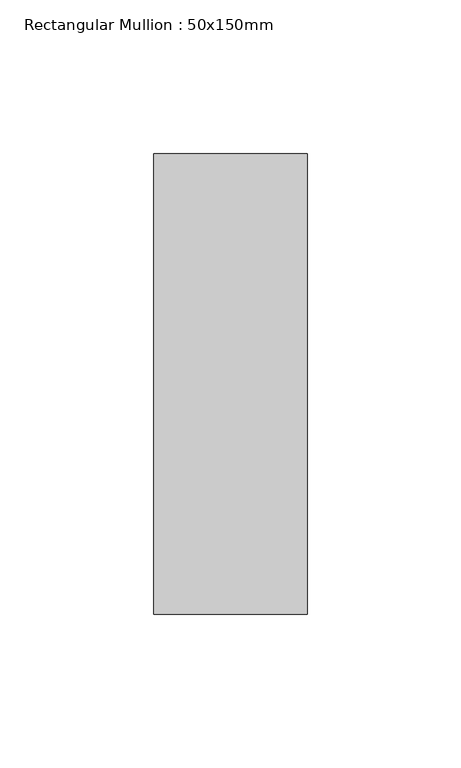
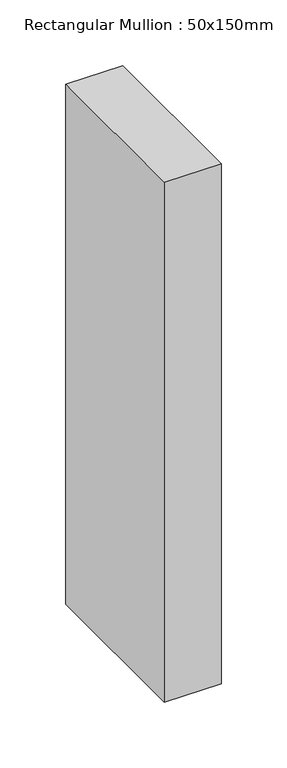
"""IFC4 building model written with IfcOpenShell, lengths in millimetres: member geometry, Rectangular Mullion : 50x150mm."""

from ifc_helpers import new_model, si_unit, frame, origin, place, context, project, spatial, polyline, outline, extrude, source, transform, mapped, element, save


def rectangular_mullion_50x150mm_b9b5507c(model_context):
    return source(origin(), model_context, "Body", "SweptSolid", [
        extrude(outline(polyline([(0.0, 75.0), (0.0, -75.0), (-50.0, -75.0), (-50.0, 75.0), (0.0, 75.0)])), frame((0.0, 0.0, -483.4), z_axis=(0.0, 0.0, 1.0), x_axis=(1.0, 0.0, 0.0)), (0.0, 0.0, 1.0), 483.4),
    ])


if __name__ == "__main__":
    model = new_model("IFC4")
    model_context = context("Model", 3, world=origin())
    ifc_project = project(units=[si_unit("LENGTHUNIT", "METRE", prefix="MILLI")], contexts=[model_context])
    site = spatial("IfcSite", under=ifc_project)
    building = spatial("IfcBuilding", under=site)
    placement = place(None, origin())
    rectangular_mullion_50x150mm_shape = rectangular_mullion_50x150mm_b9b5507c(model_context)
    element("IfcMember", 1, ObjectType="Rectangular Mullion : 50x150mm", at=placement, inside=building, context=model_context, shape_type="MappedRepresentation", body=[
        mapped(rectangular_mullion_50x150mm_shape, transform((0.0, 0.0, 0.0), x_axis=(1.0, 0.0, 0.0), y_axis=(0.0, 1.0, 0.0), z_axis=(0.0, 0.0, 1.0))),
    ])
    save(model, "model.ifc")

# Revit data of these elements
# Type "Rectangular Mullion : 50x150mm"
#   Keynote = "H11"
#   built-in parameter 1007304 = 0.492126 (stored number, unit not read)
#   built-in parameter 1007301 = 0.082021 (stored number, unit not read)
#   built-in parameter 1007300 = 0.082021 (stored number, unit not read)
# Element 1 (IfcMember, "Rectangular Mullion : 50x150mm")
#   Materials on its faces: "Aluminium"
# Materials
#   "Aluminium": class "Metal", colour RGB 247 247 247, transparency 0, Description = "Aluminium 6061", Cost = 0
